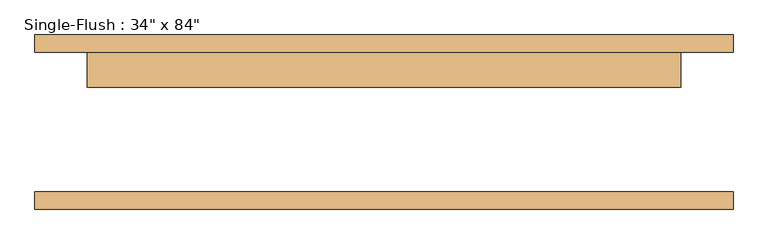
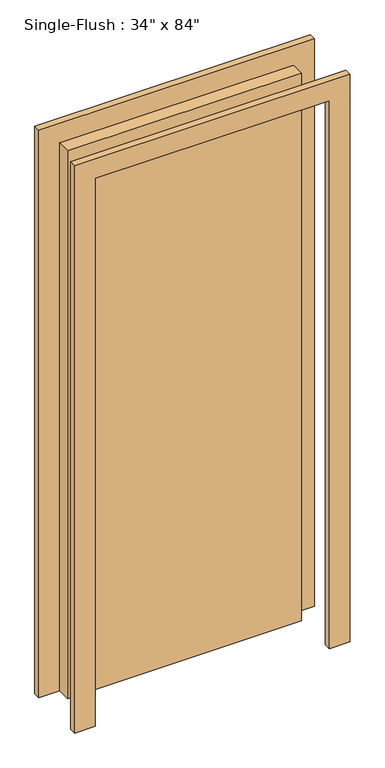
"""IFC4 building model written with IfcOpenShell, lengths in millimetres: door geometry."""

from ifc_helpers import new_model, si_unit, frame, origin, origin_with_axes, place, context, project, spatial, polyline, outline, extrude, source, transform, mapped, element, save


def door_f75d31f8(model_context):
    return source(origin(), model_context, "Body", "SweptSolid", [
        extrude(outline(polyline([(2209.8, -508.0), (0.0, -508.0), (0.0, -431.8), (2133.6, -431.8), (2133.6, 431.8), (0.0, 431.8), (0.0, 508.0), (2209.8, 508.0), (2209.8, -508.0)])), frame((0.0, 101.6, 0.0), z_axis=(0.0, 1.0, 0.0), x_axis=(0.0, 0.0, 1.0)), (0.0, 0.0, 1.0), 25.4),
        extrude(outline(polyline([(2209.8, 508.0), (2209.8, -508.0), (0.0, -508.0), (0.0, -431.8), (2133.6, -431.8), (2133.6, 431.8), (0.0, 431.8), (0.0, 508.0), (2209.8, 508.0)])), frame((0.0, -127.0, 0.0), z_axis=(0.0, 1.0, 0.0), x_axis=(0.0, 0.0, 1.0)), (0.0, 0.0, 1.0), 25.4),
        extrude(outline(polyline([(431.8, 50.8), (-431.8, 50.8), (-431.8, 101.6), (431.8, 101.6), (431.8, 50.8)])), origin_with_axes(), (0.0, 0.0, 1.0), 2133.6),
    ])


if __name__ == "__main__":
    model = new_model("IFC4")
    model_context = context("Model", 3, world=origin())
    ifc_project = project(units=[si_unit("LENGTHUNIT", "METRE", prefix="MILLI")], contexts=[model_context])
    site = spatial("IfcSite", under=ifc_project)
    building = spatial("IfcBuilding", under=site)
    placement = place(None, origin())
    door_shape = door_f75d31f8(model_context)
    element("IfcDoor", 1, ObjectType="Single-Flush : 34\" x 84\"", at=placement, inside=building, context=model_context, shape_type="MappedRepresentation", body=[
        mapped(door_shape, transform((0.0, 0.0, 0.0), x_axis=(1.0, 0.0, 0.0), y_axis=(0.0, 1.0, 0.0), z_axis=(0.0, 0.0, 1.0))),
    ])
    save(model, "model.ifc")

# Revit data of these elements
# Type "Single-Flush : 34\" x 84\""
#   Type Mark = "2"
#   Construction Type Id = "MDOOR"
#   Assembly Code = "C1020"
#   Analytic Construction = "Metal"
#   Thickness = 0' - 2"
#   Heat Transfer Coefficient (U) = 0.651978 BTU/(h·ft²·°F)
#   Height = 7' - 0"
#   Trim Projection Ext = 0' - 1"
#   Trim Projection Int = 0' - 1"
#   Trim Width = 0' - 3"
#   Width = 2' - 10"
#   Define Thermal Properties by = 1
#   Door Material = Door - Panel
#   Frame Material = Door - Frame
#   Visual Light Transmittance = 0
#   Solar Heat Gain Coefficient = 0
#   Function = (empty or 0)
#   Wall Closure = (empty or 0)
# Element 1 (IfcDoor, "Single-Flush : 34\" x 84\"")
#   Materials on its faces: "Door - Frame", "Door - Panel"
# Materials
#   "Door - Panel": class "Wood", colour RGB 210 159 95, transparency 0
#   "Door - Frame": colour RGB 118 70 51, transparency 0
